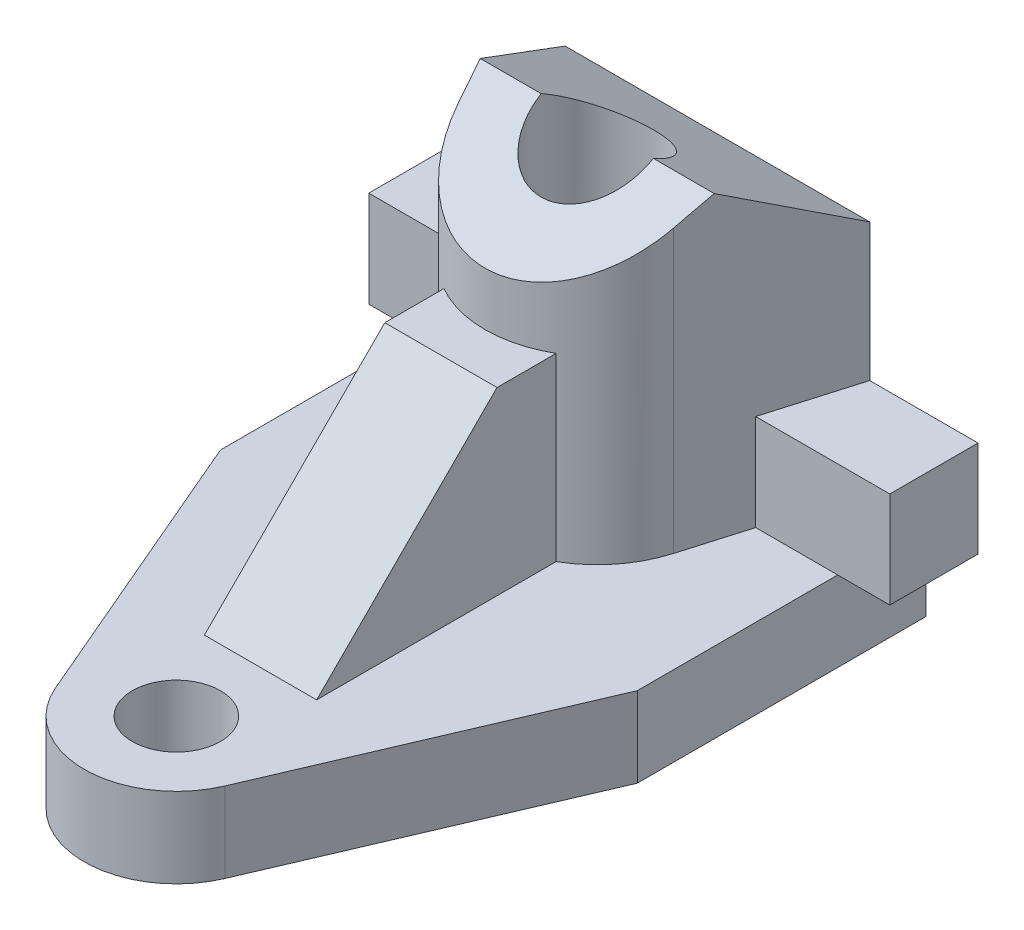
ISO-10303-21;
HEADER;
FILE_DESCRIPTION(('STEP AP214'),'2;1');
FILE_NAME('part.step','',(''),(''),'','','');
FILE_SCHEMA(('AUTOMOTIVE_DESIGN { 1 0 10303 214 1 1 1 1 }'));
ENDSEC;
DATA;
#1=APPLICATION_CONTEXT('core data for automotive mechanical design processes');
#2=APPLICATION_PROTOCOL_DEFINITION('international standard','automotive_design',2000,#1);
#3=PRODUCT_CONTEXT('',#1,'mechanical');
#4=PRODUCT('Part','Part','',(#3));
#5=PRODUCT_RELATED_PRODUCT_CATEGORY('part','',(#4));
#6=PRODUCT_DEFINITION_FORMATION('','',#4);
#7=PRODUCT_DEFINITION_CONTEXT('part definition',#1,'design');
#8=PRODUCT_DEFINITION('design','',#6,#7);
#9=PRODUCT_DEFINITION_SHAPE('','',#8);
#10=(LENGTH_UNIT() NAMED_UNIT(*) SI_UNIT(.MILLI.,.METRE.));
#11=(NAMED_UNIT(*) PLANE_ANGLE_UNIT() SI_UNIT($,.RADIAN.));
#12=(NAMED_UNIT(*) SI_UNIT($,.STERADIAN.) SOLID_ANGLE_UNIT());
#13=UNCERTAINTY_MEASURE_WITH_UNIT(LENGTH_MEASURE(1.E-05),#10,'distance_accuracy_value','');
#14=(GEOMETRIC_REPRESENTATION_CONTEXT(3) GLOBAL_UNCERTAINTY_ASSIGNED_CONTEXT((#13)) GLOBAL_UNIT_ASSIGNED_CONTEXT((#10,
#11,#12)) REPRESENTATION_CONTEXT('',''));
#15=CARTESIAN_POINT('',(0.,0.,0.));
#16=DIRECTION('',(0.,0.,1.));
#17=DIRECTION('',(1.,0.,0.));
#18=AXIS2_PLACEMENT_3D('',#15,#16,#17);
#19=CARTESIAN_POINT('',(0.,47.5,15.));
#20=DIRECTION('',(0.,-1.,0.));
#21=DIRECTION('',(0.,0.,-1.));
#22=AXIS2_PLACEMENT_3D('',#19,#20,#21);
#23=CYLINDRICAL_SURFACE('',#22,14.);
#24=DIRECTION('',(0.,-1.,0.));
#25=VECTOR('',#24,1.);
#26=CARTESIAN_POINT('',(13.432026805815,47.5,18.9472339540324));
#27=LINE('',#26,#25);
#28=CARTESIAN_POINT('',(13.432026805815,45.1417782203444,18.9472339540324));
#29=VERTEX_POINT('',#28);
#30=CARTESIAN_POINT('',(13.432026805815,10.,18.9472339540324));
#31=VERTEX_POINT('',#30);
#32=EDGE_CURVE('E324',#29,#31,#27,.T.);
#33=ORIENTED_EDGE('',*,*,#32,.F.);
#34=CARTESIAN_POINT('',(0.,47.5,15.));
#35=DIRECTION('',(0.,0.858462268371686,0.512876723767164));
#36=DIRECTION('',(0.,-0.512876723767164,0.858462268371686));
#37=AXIS2_PLACEMENT_3D('',#34,#35,#36);
#38=ELLIPSE('',#37,16.3082298614649,14.);
#39=CARTESIAN_POINT('',(-13.432026805815,45.1417782203444,18.9472339540324));
#40=VERTEX_POINT('',#39);
#41=EDGE_CURVE('E286',#40,#29,#38,.T.);
#42=ORIENTED_EDGE('',*,*,#41,.F.);
#43=DIRECTION('',(0.,-1.,0.));
#44=VECTOR('',#43,1.);
#45=CARTESIAN_POINT('',(-13.432026805815,47.5,18.9472339540324));
#46=LINE('',#45,#44);
#47=CARTESIAN_POINT('',(-13.432026805815,10.,18.9472339540324));
#48=VERTEX_POINT('',#47);
#49=EDGE_CURVE('E284',#40,#48,#46,.T.);
#50=ORIENTED_EDGE('',*,*,#49,.T.);
#51=CARTESIAN_POINT('',(0.,10.,15.));
#52=DIRECTION('',(0.,-1.,0.));
#53=DIRECTION('',(0.,0.,-1.));
#54=AXIS2_PLACEMENT_3D('',#51,#52,#53);
#55=CIRCLE('',#54,14.);
#56=CARTESIAN_POINT('',(-7.,10.,27.1243556529821));
#57=VERTEX_POINT('',#56);
#58=EDGE_CURVE('E336',#48,#57,#55,.F.);
#59=ORIENTED_EDGE('',*,*,#58,.T.);
#60=DIRECTION('',(0.,-1.,0.));
#61=VECTOR('',#60,1.);
#62=CARTESIAN_POINT('',(-7.,47.5,27.1243556529821));
#63=LINE('',#62,#61);
#64=CARTESIAN_POINT('',(-7.,32.5,27.1243556529821));
#65=VERTEX_POINT('',#64);
#66=EDGE_CURVE('E438',#57,#65,#63,.F.);
#67=ORIENTED_EDGE('',*,*,#66,.T.);
#68=CARTESIAN_POINT('',(0.,32.5,15.));
#69=DIRECTION('',(0.,-1.,0.));
#70=DIRECTION('',(0.,0.,-1.));
#71=AXIS2_PLACEMENT_3D('',#68,#69,#70);
#72=CIRCLE('',#71,14.);
#73=CARTESIAN_POINT('',(7.,32.5,27.1243556529821));
#74=VERTEX_POINT('',#73);
#75=EDGE_CURVE('E441',#74,#65,#72,.T.);
#76=ORIENTED_EDGE('',*,*,#75,.F.);
#77=DIRECTION('',(0.,-1.,0.));
#78=VECTOR('',#77,1.);
#79=CARTESIAN_POINT('',(7.,47.5,27.1243556529821));
#80=LINE('',#79,#78);
#81=CARTESIAN_POINT('',(7.,10.,27.1243556529821));
#82=VERTEX_POINT('',#81);
#83=EDGE_CURVE('E445',#82,#74,#80,.F.);
#84=ORIENTED_EDGE('',*,*,#83,.F.);
#85=EDGE_CURVE('E340',#82,#31,#55,.F.);
#86=ORIENTED_EDGE('',*,*,#85,.T.);
#87=EDGE_LOOP('',(#33,#42,#50,#59,#67,#76,#84,#86));
#88=FACE_BOUND('',#87,.T.);
#89=ADVANCED_FACE('F111',(#88),#23,.T.);
#90=CARTESIAN_POINT('',(-13.432026805815,47.5,18.9472339540324));
#91=DIRECTION('',(-0.959430486129646,0.,0.281945282430885));
#92=DIRECTION('',(0.281945282430885,0.,0.959430486129646));
#93=AXIS2_PLACEMENT_3D('',#90,#91,#92);
#94=PLANE('',#93);
#95=ORIENTED_EDGE('',*,*,#49,.F.);
#96=DIRECTION('',(-0.244610307501832,0.497296283457055,-0.832383447651177));
#97=VECTOR('',#96,1.);
#98=CARTESIAN_POINT('',(-13.7188898568264,45.724974940818,17.9710688126563));
#99=LINE('',#98,#97);
#100=CARTESIAN_POINT('',(-14.5919899381936,47.5,15.));
#101=VERTEX_POINT('',#100);
#102=EDGE_CURVE('E268',#40,#101,#99,.T.);
#103=ORIENTED_EDGE('',*,*,#102,.T.);
#104=DIRECTION('',(0.248604488500138,0.471722076970145,0.845975230368217));
#105=VECTOR('',#104,1.);
#106=CARTESIAN_POINT('',(-13.6901437947338,49.2112351368513,18.0688886736238));
#107=LINE('',#106,#105);
#108=CARTESIAN_POINT('',(-19.,39.1358884982101,0.));
#109=VERTEX_POINT('',#108);
#110=EDGE_CURVE('E282',#109,#101,#107,.T.);
#111=ORIENTED_EDGE('',*,*,#110,.F.);
#112=DIRECTION('',(0.,-1.,0.));
#113=VECTOR('',#112,1.);
#114=CARTESIAN_POINT('',(-19.,47.5,0.));
#115=LINE('',#114,#113);
#116=CARTESIAN_POINT('',(-19.,22.,0.));
#117=VERTEX_POINT('',#116);
#118=EDGE_CURVE('E322',#109,#117,#115,.T.);
#119=ORIENTED_EDGE('',*,*,#118,.T.);
#120=DIRECTION('',(0.281945282430885,0.,0.959430486129646));
#121=VECTOR('',#120,1.);
#122=CARTESIAN_POINT('',(-17.4896302965844,22.,5.13963108830785));
#123=LINE('',#122,#121);
#124=CARTESIAN_POINT('',(-15.7674592880087,22.,11.));
#125=VERTEX_POINT('',#124);
#126=EDGE_CURVE('E436',#117,#125,#123,.T.);
#127=ORIENTED_EDGE('',*,*,#126,.T.);
#128=DIRECTION('',(0.,1.,0.));
#129=VECTOR('',#128,1.);
#130=CARTESIAN_POINT('',(-15.7674592880087,22.,11.));
#131=LINE('',#130,#129);
#132=CARTESIAN_POINT('',(-15.7674592880087,10.,11.));
#133=VERTEX_POINT('',#132);
#134=EDGE_CURVE('E331',#133,#125,#131,.T.);
#135=ORIENTED_EDGE('',*,*,#134,.F.);
#136=DIRECTION('',(-0.281945282430885,0.,-0.959430486129646));
#137=VECTOR('',#136,1.);
#138=CARTESIAN_POINT('',(0.769585411877711,10.,67.2738439840683));
#139=LINE('',#138,#137);
#140=EDGE_CURVE('E333',#48,#133,#139,.T.);
#141=ORIENTED_EDGE('',*,*,#140,.F.);
#142=EDGE_LOOP('',(#95,#103,#111,#119,#127,#135,#141));
#143=FACE_BOUND('',#142,.T.);
#144=ADVANCED_FACE('F278',(#143),#94,.T.);
#145=CARTESIAN_POINT('',(13.432026805815,47.5,18.9472339540324));
#146=DIRECTION('',(-0.959430486129646,0.,-0.281945282430885));
#147=DIRECTION('',(-0.281945282430885,0.,0.959430486129646));
#148=AXIS2_PLACEMENT_3D('',#145,#146,#147);
#149=PLANE('',#148);
#150=DIRECTION('',(0.244610307501832,0.497296283457055,-0.832383447651177));
#151=VECTOR('',#150,1.);
#152=CARTESIAN_POINT('',(13.7188898568264,45.724974940818,17.9710688126563));
#153=LINE('',#152,#151);
#154=CARTESIAN_POINT('',(14.5919899381936,47.5,15.));
#155=VERTEX_POINT('',#154);
#156=EDGE_CURVE('E452',#29,#155,#153,.T.);
#157=ORIENTED_EDGE('',*,*,#156,.F.);
#158=ORIENTED_EDGE('',*,*,#32,.T.);
#159=DIRECTION('',(0.281945282430885,0.,-0.959430486129646));
#160=VECTOR('',#159,1.);
#161=CARTESIAN_POINT('',(-0.769585411877739,10.,67.2738439840683));
#162=LINE('',#161,#160);
#163=CARTESIAN_POINT('',(15.7674592880086,10.,11.));
#164=VERTEX_POINT('',#163);
#165=EDGE_CURVE('E329',#31,#164,#162,.T.);
#166=ORIENTED_EDGE('',*,*,#165,.T.);
#167=DIRECTION('',(0.,1.,0.));
#168=VECTOR('',#167,1.);
#169=CARTESIAN_POINT('',(15.7674592880086,22.,11.));
#170=LINE('',#169,#168);
#171=CARTESIAN_POINT('',(15.7674592880086,22.,11.));
#172=VERTEX_POINT('',#171);
#173=EDGE_CURVE('E136',#164,#172,#170,.T.);
#174=ORIENTED_EDGE('',*,*,#173,.T.);
#175=DIRECTION('',(-0.281945282430885,0.,0.959430486129646));
#176=VECTOR('',#175,1.);
#177=CARTESIAN_POINT('',(17.4896302965844,22.,5.13963108830785));
#178=LINE('',#177,#176);
#179=CARTESIAN_POINT('',(19.,22.,0.));
#180=VERTEX_POINT('',#179);
#181=EDGE_CURVE('E432',#180,#172,#178,.T.);
#182=ORIENTED_EDGE('',*,*,#181,.F.);
#183=DIRECTION('',(0.,-1.,0.));
#184=VECTOR('',#183,1.);
#185=CARTESIAN_POINT('',(19.,47.5,0.));
#186=LINE('',#185,#184);
#187=CARTESIAN_POINT('',(19.,39.1358884982101,0.));
#188=VERTEX_POINT('',#187);
#189=EDGE_CURVE('E323',#188,#180,#186,.T.);
#190=ORIENTED_EDGE('',*,*,#189,.F.);
#191=DIRECTION('',(-0.248604488500138,0.471722076970145,0.845975230368217));
#192=VECTOR('',#191,1.);
#193=CARTESIAN_POINT('',(13.6901437947338,49.2112351368513,18.0688886736238));
#194=LINE('',#193,#192);
#195=EDGE_CURVE('E293',#188,#155,#194,.T.);
#196=ORIENTED_EDGE('',*,*,#195,.T.);
#197=EDGE_LOOP('',(#157,#158,#166,#174,#182,#190,#196));
#198=FACE_BOUND('',#197,.T.);
#199=ADVANCED_FACE('F460',(#198),#149,.F.);
#200=CARTESIAN_POINT('',(0.,47.5,15.));
#201=DIRECTION('',(0.,-1.,0.));
#202=DIRECTION('',(0.,0.,-1.));
#203=AXIS2_PLACEMENT_3D('',#200,#201,#202);
#204=CYLINDRICAL_SURFACE('',#203,7.);
#205=CARTESIAN_POINT('',(0.,15.,15.));
#206=DIRECTION('',(0.,1.,0.));
#207=DIRECTION('',(0.,0.,1.));
#208=AXIS2_PLACEMENT_3D('',#205,#206,#207);
#209=CIRCLE('',#208,7.);
#210=CARTESIAN_POINT('',(0.,15.,22.));
#211=VERTEX_POINT('',#210);
#212=EDGE_CURVE('E114',#211,#211,#209,.T.);
#213=ORIENTED_EDGE('',*,*,#212,.F.);
#214=EDGE_LOOP('',(#213));
#215=FACE_BOUND('',#214,.T.);
#216=CARTESIAN_POINT('',(0.,47.5,15.));
#217=DIRECTION('',(0.,-0.873395405977944,0.487011770716707));
#218=DIRECTION('',(0.,-0.487011770716707,-0.873395405977944));
#219=AXIS2_PLACEMENT_3D('',#216,#217,#218);
#220=ELLIPSE('',#219,8.01469752655966,7.);
#221=CARTESIAN_POINT('',(-7.,47.5,15.));
#222=VERTEX_POINT('',#221);
#223=CARTESIAN_POINT('',(7.,47.5,15.));
#224=VERTEX_POINT('',#223);
#225=EDGE_CURVE('E300',#222,#224,#220,.T.);
#226=ORIENTED_EDGE('',*,*,#225,.F.);
#227=CARTESIAN_POINT('',(0.,47.5,15.));
#228=DIRECTION('',(0.,0.858462268371686,0.512876723767164));
#229=DIRECTION('',(0.,-0.512876723767164,0.858462268371686));
#230=AXIS2_PLACEMENT_3D('',#227,#228,#229);
#231=ELLIPSE('',#230,8.15411493073244,7.);
#232=EDGE_CURVE('E275',#222,#224,#231,.T.);
#233=ORIENTED_EDGE('',*,*,#232,.T.);
#234=EDGE_LOOP('',(#226,#233));
#235=FACE_BOUND('',#234,.T.);
#236=ADVANCED_FACE('F448',(#215,#235),#204,.F.);
#237=CARTESIAN_POINT('',(-26.,10.,0.));
#238=DIRECTION('',(0.,0.,-1.));
#239=DIRECTION('',(-1.,0.,0.));
#240=AXIS2_PLACEMENT_3D('',#237,#238,#239);
#241=PLANE('',#240);
#242=ORIENTED_EDGE('',*,*,#118,.F.);
#243=DIRECTION('',(1.,0.,0.));
#244=VECTOR('',#243,1.);
#245=CARTESIAN_POINT('',(-32.5,39.1358884982101,0.));
#246=LINE('',#245,#244);
#247=EDGE_CURVE('E281',#109,#188,#246,.T.);
#248=ORIENTED_EDGE('',*,*,#247,.T.);
#249=ORIENTED_EDGE('',*,*,#189,.T.);
#250=DIRECTION('',(-1.,0.,0.));
#251=VECTOR('',#250,1.);
#252=CARTESIAN_POINT('',(-32.5,22.,0.));
#253=LINE('',#252,#251);
#254=CARTESIAN_POINT('',(32.5,22.,0.));
#255=VERTEX_POINT('',#254);
#256=EDGE_CURVE('E352',#255,#180,#253,.T.);
#257=ORIENTED_EDGE('',*,*,#256,.F.);
#258=DIRECTION('',(0.,-1.,0.));
#259=VECTOR('',#258,1.);
#260=CARTESIAN_POINT('',(32.5,22.,0.));
#261=LINE('',#260,#259);
#262=CARTESIAN_POINT('',(32.5,10.,0.));
#263=VERTEX_POINT('',#262);
#264=EDGE_CURVE('E375',#255,#263,#261,.T.);
#265=ORIENTED_EDGE('',*,*,#264,.T.);
#266=DIRECTION('',(-1.,0.,0.));
#267=VECTOR('',#266,1.);
#268=CARTESIAN_POINT('',(-32.5,10.,0.));
#269=LINE('',#268,#267);
#270=CARTESIAN_POINT('',(26.,10.,0.));
#271=VERTEX_POINT('',#270);
#272=EDGE_CURVE('E347',#263,#271,#269,.T.);
#273=ORIENTED_EDGE('',*,*,#272,.T.);
#274=DIRECTION('',(0.,-1.,0.));
#275=VECTOR('',#274,1.);
#276=CARTESIAN_POINT('',(26.,10.,0.));
#277=LINE('',#276,#275);
#278=CARTESIAN_POINT('',(26.,0.,0.));
#279=VERTEX_POINT('',#278);
#280=EDGE_CURVE('E422',#271,#279,#277,.T.);
#281=ORIENTED_EDGE('',*,*,#280,.T.);
#282=DIRECTION('',(1.,0.,0.));
#283=VECTOR('',#282,1.);
#284=CARTESIAN_POINT('',(-26.,0.,0.));
#285=LINE('',#284,#283);
#286=CARTESIAN_POINT('',(-26.,0.,0.));
#287=VERTEX_POINT('',#286);
#288=EDGE_CURVE('E418',#287,#279,#285,.T.);
#289=ORIENTED_EDGE('',*,*,#288,.F.);
#290=DIRECTION('',(0.,-1.,0.));
#291=VECTOR('',#290,1.);
#292=CARTESIAN_POINT('',(-26.,10.,0.));
#293=LINE('',#292,#291);
#294=CARTESIAN_POINT('',(-26.,10.,0.));
#295=VERTEX_POINT('',#294);
#296=EDGE_CURVE('E404',#295,#287,#293,.T.);
#297=ORIENTED_EDGE('',*,*,#296,.F.);
#298=CARTESIAN_POINT('',(-32.5,10.,0.));
#299=VERTEX_POINT('',#298);
#300=EDGE_CURVE('E370',#295,#299,#269,.T.);
#301=ORIENTED_EDGE('',*,*,#300,.T.);
#302=DIRECTION('',(0.,-1.,0.));
#303=VECTOR('',#302,1.);
#304=CARTESIAN_POINT('',(-32.5,22.,0.));
#305=LINE('',#304,#303);
#306=CARTESIAN_POINT('',(-32.5,22.,0.));
#307=VERTEX_POINT('',#306);
#308=EDGE_CURVE('E358',#307,#299,#305,.T.);
#309=ORIENTED_EDGE('',*,*,#308,.F.);
#310=EDGE_CURVE('E355',#117,#307,#253,.T.);
#311=ORIENTED_EDGE('',*,*,#310,.F.);
#312=EDGE_LOOP('',(#242,#248,#249,#257,#265,#273,#281,#289,#297,#301,#309,#311));
#313=FACE_BOUND('',#312,.T.);
#314=ADVANCED_FACE('F479',(#313),#241,.T.);
#315=CARTESIAN_POINT('',(0.,10.,67.5));
#316=DIRECTION('',(0.,-1.,0.));
#317=DIRECTION('',(0.,0.,-1.));
#318=AXIS2_PLACEMENT_3D('',#315,#316,#317);
#319=PLANE('',#318);
#320=DIRECTION('',(-1.,0.,0.));
#321=VECTOR('',#320,1.);
#322=CARTESIAN_POINT('',(7.,10.,57.));
#323=LINE('',#322,#321);
#324=CARTESIAN_POINT('',(7.,10.,57.));
#325=VERTEX_POINT('',#324);
#326=CARTESIAN_POINT('',(-7.,10.,57.));
#327=VERTEX_POINT('',#326);
#328=EDGE_CURVE('E309',#325,#327,#323,.T.);
#329=ORIENTED_EDGE('',*,*,#328,.T.);
#330=DIRECTION('',(0.,0.,-1.));
#331=VECTOR('',#330,1.);
#332=CARTESIAN_POINT('',(-7.,10.,26.5));
#333=LINE('',#332,#331);
#334=EDGE_CURVE('E311',#327,#57,#333,.T.);
#335=ORIENTED_EDGE('',*,*,#334,.T.);
#336=ORIENTED_EDGE('',*,*,#58,.F.);
#337=ORIENTED_EDGE('',*,*,#140,.T.);
#338=DIRECTION('',(1.,0.,0.));
#339=VECTOR('',#338,1.);
#340=CARTESIAN_POINT('',(-32.5,10.,11.));
#341=LINE('',#340,#339);
#342=CARTESIAN_POINT('',(-26.,10.,11.));
#343=VERTEX_POINT('',#342);
#344=EDGE_CURVE('E362',#343,#133,#341,.T.);
#345=ORIENTED_EDGE('',*,*,#344,.F.);
#346=DIRECTION('',(0.,0.,1.));
#347=VECTOR('',#346,1.);
#348=CARTESIAN_POINT('',(-26.,10.,0.));
#349=LINE('',#348,#347);
#350=CARTESIAN_POINT('',(-26.,10.,36.));
#351=VERTEX_POINT('',#350);
#352=EDGE_CURVE('E395',#343,#351,#349,.T.);
#353=ORIENTED_EDGE('',*,*,#352,.T.);
#354=DIRECTION('',(0.393668654576833,0.,0.919252408429625));
#355=VECTOR('',#354,1.);
#356=CARTESIAN_POINT('',(-26.,10.,36.));
#357=LINE('',#356,#355);
#358=CARTESIAN_POINT('',(-10.5714026969407,10.,72.0271895276336));
#359=VERTEX_POINT('',#358);
#360=EDGE_CURVE('E392',#351,#359,#357,.T.);
#361=ORIENTED_EDGE('',*,*,#360,.T.);
#362=CARTESIAN_POINT('',(0.,10.,67.5));
#363=DIRECTION('',(0.,-1.,0.));
#364=DIRECTION('',(0.,0.,-1.));
#365=AXIS2_PLACEMENT_3D('',#362,#363,#364);
#366=CIRCLE('',#365,11.5);
#367=CARTESIAN_POINT('',(10.5714026969407,10.,72.0271895276336));
#368=VERTEX_POINT('',#367);
#369=EDGE_CURVE('E394',#368,#359,#366,.T.);
#370=ORIENTED_EDGE('',*,*,#369,.F.);
#371=DIRECTION('',(-0.393668654576833,0.,0.919252408429625));
#372=VECTOR('',#371,1.);
#373=CARTESIAN_POINT('',(26.,10.,36.));
#374=LINE('',#373,#372);
#375=CARTESIAN_POINT('',(26.,10.,36.));
#376=VERTEX_POINT('',#375);
#377=EDGE_CURVE('E400',#376,#368,#374,.T.);
#378=ORIENTED_EDGE('',*,*,#377,.F.);
#379=DIRECTION('',(0.,0.,1.));
#380=VECTOR('',#379,1.);
#381=CARTESIAN_POINT('',(26.,10.,0.));
#382=LINE('',#381,#380);
#383=CARTESIAN_POINT('',(26.,10.,11.));
#384=VERTEX_POINT('',#383);
#385=EDGE_CURVE('E399',#384,#376,#382,.T.);
#386=ORIENTED_EDGE('',*,*,#385,.F.);
#387=EDGE_CURVE('E364',#164,#384,#341,.T.);
#388=ORIENTED_EDGE('',*,*,#387,.F.);
#389=ORIENTED_EDGE('',*,*,#165,.F.);
#390=ORIENTED_EDGE('',*,*,#85,.F.);
#391=DIRECTION('',(0.,0.,-1.));
#392=VECTOR('',#391,1.);
#393=CARTESIAN_POINT('',(7.,10.,26.5));
#394=LINE('',#393,#392);
#395=EDGE_CURVE('E303',#325,#82,#394,.T.);
#396=ORIENTED_EDGE('',*,*,#395,.F.);
#397=EDGE_LOOP('',(#329,#335,#336,#337,#345,#353,#361,#370,#378,#386,#388,#389,#390,#396));
#398=FACE_BOUND('',#397,.T.);
#399=CARTESIAN_POINT('',(0.,10.,67.5));
#400=DIRECTION('',(0.,-1.,0.));
#401=DIRECTION('',(0.,0.,-1.));
#402=AXIS2_PLACEMENT_3D('',#399,#400,#401);
#403=CIRCLE('',#402,5.5);
#404=CARTESIAN_POINT('',(0.,10.,62.));
#405=VERTEX_POINT('',#404);
#406=EDGE_CURVE('E385',#405,#405,#403,.T.);
#407=ORIENTED_EDGE('',*,*,#406,.T.);
#408=EDGE_LOOP('',(#407));
#409=FACE_BOUND('',#408,.T.);
#410=ADVANCED_FACE('F467',(#398,#409),#319,.F.);
#411=CARTESIAN_POINT('',(-32.5,22.,11.));
#412=DIRECTION('',(0.,0.,-1.));
#413=DIRECTION('',(-1.,0.,0.));
#414=AXIS2_PLACEMENT_3D('',#411,#412,#413);
#415=PLANE('',#414);
#416=ORIENTED_EDGE('',*,*,#173,.F.);
#417=ORIENTED_EDGE('',*,*,#387,.T.);
#418=CARTESIAN_POINT('',(32.5,10.,11.));
#419=VERTEX_POINT('',#418);
#420=EDGE_CURVE('E360',#384,#419,#341,.T.);
#421=ORIENTED_EDGE('',*,*,#420,.T.);
#422=DIRECTION('',(0.,-1.,0.));
#423=VECTOR('',#422,1.);
#424=CARTESIAN_POINT('',(32.5,22.,11.));
#425=LINE('',#424,#423);
#426=CARTESIAN_POINT('',(32.5,22.,11.));
#427=VERTEX_POINT('',#426);
#428=EDGE_CURVE('E374',#427,#419,#425,.T.);
#429=ORIENTED_EDGE('',*,*,#428,.F.);
#430=DIRECTION('',(1.,0.,0.));
#431=VECTOR('',#430,1.);
#432=CARTESIAN_POINT('',(-32.5,22.,11.));
#433=LINE('',#432,#431);
#434=EDGE_CURVE('E343',#172,#427,#433,.T.);
#435=ORIENTED_EDGE('',*,*,#434,.F.);
#436=EDGE_LOOP('',(#416,#417,#421,#429,#435));
#437=FACE_BOUND('',#436,.T.);
#438=ADVANCED_FACE('F472',(#437),#415,.F.);
#439=ORIENTED_EDGE('',*,*,#344,.T.);
#440=ORIENTED_EDGE('',*,*,#134,.T.);
#441=CARTESIAN_POINT('',(-32.5,22.,11.));
#442=VERTEX_POINT('',#441);
#443=EDGE_CURVE('E350',#442,#125,#433,.T.);
#444=ORIENTED_EDGE('',*,*,#443,.F.);
#445=DIRECTION('',(0.,-1.,0.));
#446=VECTOR('',#445,1.);
#447=CARTESIAN_POINT('',(-32.5,22.,11.));
#448=LINE('',#447,#446);
#449=CARTESIAN_POINT('',(-32.5,10.,11.));
#450=VERTEX_POINT('',#449);
#451=EDGE_CURVE('E377',#442,#450,#448,.T.);
#452=ORIENTED_EDGE('',*,*,#451,.T.);
#453=EDGE_CURVE('E359',#450,#343,#341,.T.);
#454=ORIENTED_EDGE('',*,*,#453,.T.);
#455=EDGE_LOOP('',(#439,#440,#444,#452,#454));
#456=FACE_BOUND('',#455,.T.);
#457=ADVANCED_FACE('F490',(#456),#415,.F.);
#458=CARTESIAN_POINT('',(0.,22.,0.));
#459=DIRECTION('',(0.,1.,0.));
#460=DIRECTION('',(0.,0.,1.));
#461=AXIS2_PLACEMENT_3D('',#458,#459,#460);
#462=PLANE('',#461);
#463=ORIENTED_EDGE('',*,*,#126,.F.);
#464=ORIENTED_EDGE('',*,*,#310,.T.);
#465=DIRECTION('',(0.,0.,1.));
#466=VECTOR('',#465,1.);
#467=CARTESIAN_POINT('',(-32.5,22.,0.));
#468=LINE('',#467,#466);
#469=EDGE_CURVE('E345',#307,#442,#468,.T.);
#470=ORIENTED_EDGE('',*,*,#469,.T.);
#471=ORIENTED_EDGE('',*,*,#443,.T.);
#472=EDGE_LOOP('',(#463,#464,#470,#471));
#473=FACE_BOUND('',#472,.T.);
#474=ADVANCED_FACE('F483',(#473),#462,.T.);
#475=CARTESIAN_POINT('',(-26.,10.,0.));
#476=DIRECTION('',(1.,0.,0.));
#477=DIRECTION('',(0.,0.,-1.));
#478=AXIS2_PLACEMENT_3D('',#475,#476,#477);
#479=PLANE('',#478);
#480=DIRECTION('',(0.,0.,1.));
#481=VECTOR('',#480,1.);
#482=CARTESIAN_POINT('',(-26.,0.,0.));
#483=LINE('',#482,#481);
#484=CARTESIAN_POINT('',(-26.,0.,36.));
#485=VERTEX_POINT('',#484);
#486=EDGE_CURVE('E383',#287,#485,#483,.T.);
#487=ORIENTED_EDGE('',*,*,#486,.T.);
#488=DIRECTION('',(0.,-1.,0.));
#489=VECTOR('',#488,1.);
#490=CARTESIAN_POINT('',(-26.,10.,36.));
#491=LINE('',#490,#489);
#492=EDGE_CURVE('E431',#351,#485,#491,.T.);
#493=ORIENTED_EDGE('',*,*,#492,.F.);
#494=ORIENTED_EDGE('',*,*,#352,.F.);
#495=EDGE_CURVE('E389',#295,#343,#349,.T.);
#496=ORIENTED_EDGE('',*,*,#495,.F.);
#497=ORIENTED_EDGE('',*,*,#296,.T.);
#498=EDGE_LOOP('',(#487,#493,#494,#496,#497));
#499=FACE_BOUND('',#498,.T.);
#500=ADVANCED_FACE('F113',(#499),#479,.F.);
#501=CARTESIAN_POINT('',(-26.,10.,36.));
#502=DIRECTION('',(0.919252408429625,0.,-0.393668654576833));
#503=DIRECTION('',(-0.393668654576833,0.,-0.919252408429625));
#504=AXIS2_PLACEMENT_3D('',#501,#502,#503);
#505=PLANE('',#504);
#506=DIRECTION('',(0.393668654576833,0.,0.919252408429625));
#507=VECTOR('',#506,1.);
#508=CARTESIAN_POINT('',(-26.,0.,36.));
#509=LINE('',#508,#507);
#510=CARTESIAN_POINT('',(-10.5714026969407,0.,72.0271895276336));
#511=VERTEX_POINT('',#510);
#512=EDGE_CURVE('E410',#485,#511,#509,.T.);
#513=ORIENTED_EDGE('',*,*,#512,.T.);
#514=DIRECTION('',(0.,-1.,0.));
#515=VECTOR('',#514,1.);
#516=CARTESIAN_POINT('',(-10.5714026969407,10.,72.0271895276336));
#517=LINE('',#516,#515);
#518=EDGE_CURVE('E429',#359,#511,#517,.T.);
#519=ORIENTED_EDGE('',*,*,#518,.F.);
#520=ORIENTED_EDGE('',*,*,#360,.F.);
#521=ORIENTED_EDGE('',*,*,#492,.T.);
#522=EDGE_LOOP('',(#513,#519,#520,#521));
#523=FACE_BOUND('',#522,.T.);
#524=ADVANCED_FACE('F557',(#523),#505,.F.);
#525=CARTESIAN_POINT('',(0.,10.,67.5));
#526=DIRECTION('',(0.,-1.,0.));
#527=DIRECTION('',(0.,0.,-1.));
#528=AXIS2_PLACEMENT_3D('',#525,#526,#527);
#529=CYLINDRICAL_SURFACE('',#528,11.5);
#530=CARTESIAN_POINT('',(0.,0.,67.5));
#531=DIRECTION('',(0.,-1.,0.));
#532=DIRECTION('',(0.,0.,-1.));
#533=AXIS2_PLACEMENT_3D('',#530,#531,#532);
#534=CIRCLE('',#533,11.5);
#535=CARTESIAN_POINT('',(10.5714026969407,0.,72.0271895276336));
#536=VERTEX_POINT('',#535);
#537=EDGE_CURVE('E408',#536,#511,#534,.T.);
#538=ORIENTED_EDGE('',*,*,#537,.F.);
#539=DIRECTION('',(0.,-1.,0.));
#540=VECTOR('',#539,1.);
#541=CARTESIAN_POINT('',(10.5714026969407,10.,72.0271895276336));
#542=LINE('',#541,#540);
#543=EDGE_CURVE('E430',#368,#536,#542,.T.);
#544=ORIENTED_EDGE('',*,*,#543,.F.);
#545=ORIENTED_EDGE('',*,*,#369,.T.);
#546=ORIENTED_EDGE('',*,*,#518,.T.);
#547=EDGE_LOOP('',(#538,#544,#545,#546));
#548=FACE_BOUND('',#547,.T.);
#549=ADVANCED_FACE('F560',(#548),#529,.T.);
#550=CARTESIAN_POINT('',(26.,10.,36.));
#551=DIRECTION('',(0.919252408429625,0.,0.393668654576833));
#552=DIRECTION('',(0.393668654576833,0.,-0.919252408429625));
#553=AXIS2_PLACEMENT_3D('',#550,#551,#552);
#554=PLANE('',#553);
#555=DIRECTION('',(-0.393668654576833,0.,0.919252408429625));
#556=VECTOR('',#555,1.);
#557=CARTESIAN_POINT('',(26.,0.,36.));
#558=LINE('',#557,#556);
#559=CARTESIAN_POINT('',(26.,0.,36.));
#560=VERTEX_POINT('',#559);
#561=EDGE_CURVE('E413',#560,#536,#558,.T.);
#562=ORIENTED_EDGE('',*,*,#561,.F.);
#563=DIRECTION('',(0.,-1.,0.));
#564=VECTOR('',#563,1.);
#565=CARTESIAN_POINT('',(26.,10.,36.));
#566=LINE('',#565,#564);
#567=EDGE_CURVE('E424',#376,#560,#566,.T.);
#568=ORIENTED_EDGE('',*,*,#567,.F.);
#569=ORIENTED_EDGE('',*,*,#377,.T.);
#570=ORIENTED_EDGE('',*,*,#543,.T.);
#571=EDGE_LOOP('',(#562,#568,#569,#570));
#572=FACE_BOUND('',#571,.T.);
#573=ADVANCED_FACE('F551',(#572),#554,.T.);
#574=CARTESIAN_POINT('',(26.,10.,0.));
#575=DIRECTION('',(1.,0.,0.));
#576=DIRECTION('',(0.,0.,-1.));
#577=AXIS2_PLACEMENT_3D('',#574,#575,#576);
#578=PLANE('',#577);
#579=DIRECTION('',(0.,0.,1.));
#580=VECTOR('',#579,1.);
#581=CARTESIAN_POINT('',(26.,0.,0.));
#582=LINE('',#581,#580);
#583=EDGE_CURVE('E416',#279,#560,#582,.T.);
#584=ORIENTED_EDGE('',*,*,#583,.F.);
#585=ORIENTED_EDGE('',*,*,#280,.F.);
#586=EDGE_CURVE('E402',#271,#384,#382,.T.);
#587=ORIENTED_EDGE('',*,*,#586,.T.);
#588=ORIENTED_EDGE('',*,*,#385,.T.);
#589=ORIENTED_EDGE('',*,*,#567,.T.);
#590=EDGE_LOOP('',(#584,#585,#587,#588,#589));
#591=FACE_BOUND('',#590,.T.);
#592=ADVANCED_FACE('F550',(#591),#578,.T.);
#593=CARTESIAN_POINT('',(0.,0.,67.5));
#594=DIRECTION('',(0.,-1.,0.));
#595=DIRECTION('',(0.,0.,-1.));
#596=AXIS2_PLACEMENT_3D('',#593,#594,#595);
#597=PLANE('',#596);
#598=CARTESIAN_POINT('',(0.,0.,15.));
#599=DIRECTION('',(0.,1.,0.));
#600=DIRECTION('',(0.,0.,1.));
#601=AXIS2_PLACEMENT_3D('',#598,#599,#600);
#602=CIRCLE('',#601,10.);
#603=CARTESIAN_POINT('',(0.,0.,25.));
#604=VERTEX_POINT('',#603);
#605=EDGE_CURVE('E289',#604,#604,#602,.T.);
#606=ORIENTED_EDGE('',*,*,#605,.T.);
#607=EDGE_LOOP('',(#606));
#608=FACE_BOUND('',#607,.T.);
#609=ORIENTED_EDGE('',*,*,#288,.T.);
#610=ORIENTED_EDGE('',*,*,#583,.T.);
#611=ORIENTED_EDGE('',*,*,#561,.T.);
#612=ORIENTED_EDGE('',*,*,#537,.T.);
#613=ORIENTED_EDGE('',*,*,#512,.F.);
#614=ORIENTED_EDGE('',*,*,#486,.F.);
#615=EDGE_LOOP('',(#609,#610,#611,#612,#613,#614));
#616=FACE_BOUND('',#615,.T.);
#617=CARTESIAN_POINT('',(0.,0.,67.5));
#618=DIRECTION('',(0.,-1.,0.));
#619=DIRECTION('',(0.,0.,-1.));
#620=AXIS2_PLACEMENT_3D('',#617,#618,#619);
#621=CIRCLE('',#620,5.5);
#622=CARTESIAN_POINT('',(0.,0.,62.));
#623=VERTEX_POINT('',#622);
#624=EDGE_CURVE('E382',#623,#623,#621,.T.);
#625=ORIENTED_EDGE('',*,*,#624,.F.);
#626=EDGE_LOOP('',(#625));
#627=FACE_BOUND('',#626,.T.);
#628=ADVANCED_FACE('F545',(#608,#616,#627),#597,.T.);
#629=CARTESIAN_POINT('',(0.,10.,67.5));
#630=DIRECTION('',(0.,-1.,0.));
#631=DIRECTION('',(0.,0.,-1.));
#632=AXIS2_PLACEMENT_3D('',#629,#630,#631);
#633=CYLINDRICAL_SURFACE('',#632,5.5);
#634=ORIENTED_EDGE('',*,*,#406,.F.);
#635=EDGE_LOOP('',(#634));
#636=FACE_BOUND('',#635,.T.);
#637=ORIENTED_EDGE('',*,*,#624,.T.);
#638=EDGE_LOOP('',(#637));
#639=FACE_BOUND('',#638,.T.);
#640=ADVANCED_FACE('F536',(#636,#639),#633,.F.);
#641=CARTESIAN_POINT('',(0.,10.,0.));
#642=DIRECTION('',(0.,1.,0.));
#643=DIRECTION('',(0.,0.,1.));
#644=AXIS2_PLACEMENT_3D('',#641,#642,#643);
#645=PLANE('',#644);
#646=ORIENTED_EDGE('',*,*,#300,.F.);
#647=ORIENTED_EDGE('',*,*,#495,.T.);
#648=ORIENTED_EDGE('',*,*,#453,.F.);
#649=DIRECTION('',(0.,0.,1.));
#650=VECTOR('',#649,1.);
#651=CARTESIAN_POINT('',(-32.5,10.,0.));
#652=LINE('',#651,#650);
#653=EDGE_CURVE('E342',#299,#450,#652,.T.);
#654=ORIENTED_EDGE('',*,*,#653,.F.);
#655=EDGE_LOOP('',(#646,#647,#648,#654));
#656=FACE_BOUND('',#655,.T.);
#657=ADVANCED_FACE('F514',(#656),#645,.F.);
#658=CARTESIAN_POINT('',(-32.5,22.,0.));
#659=DIRECTION('',(1.,0.,0.));
#660=DIRECTION('',(0.,0.,-1.));
#661=AXIS2_PLACEMENT_3D('',#658,#659,#660);
#662=PLANE('',#661);
#663=ORIENTED_EDGE('',*,*,#653,.T.);
#664=ORIENTED_EDGE('',*,*,#451,.F.);
#665=ORIENTED_EDGE('',*,*,#469,.F.);
#666=ORIENTED_EDGE('',*,*,#308,.T.);
#667=EDGE_LOOP('',(#663,#664,#665,#666));
#668=FACE_BOUND('',#667,.T.);
#669=ADVANCED_FACE('F535',(#668),#662,.F.);
#670=CARTESIAN_POINT('',(32.5,22.,0.));
#671=DIRECTION('',(-1.,0.,0.));
#672=DIRECTION('',(0.,0.,1.));
#673=AXIS2_PLACEMENT_3D('',#670,#671,#672);
#674=PLANE('',#673);
#675=DIRECTION('',(0.,0.,-1.));
#676=VECTOR('',#675,1.);
#677=CARTESIAN_POINT('',(32.5,10.,0.));
#678=LINE('',#677,#676);
#679=EDGE_CURVE('E361',#419,#263,#678,.T.);
#680=ORIENTED_EDGE('',*,*,#679,.T.);
#681=ORIENTED_EDGE('',*,*,#264,.F.);
#682=DIRECTION('',(0.,0.,-1.));
#683=VECTOR('',#682,1.);
#684=CARTESIAN_POINT('',(32.5,22.,0.));
#685=LINE('',#684,#683);
#686=EDGE_CURVE('E346',#427,#255,#685,.T.);
#687=ORIENTED_EDGE('',*,*,#686,.F.);
#688=ORIENTED_EDGE('',*,*,#428,.T.);
#689=EDGE_LOOP('',(#680,#681,#687,#688));
#690=FACE_BOUND('',#689,.T.);
#691=ADVANCED_FACE('F527',(#690),#674,.F.);
#692=ORIENTED_EDGE('',*,*,#256,.T.);
#693=ORIENTED_EDGE('',*,*,#181,.T.);
#694=ORIENTED_EDGE('',*,*,#434,.T.);
#695=ORIENTED_EDGE('',*,*,#686,.T.);
#696=EDGE_LOOP('',(#692,#693,#694,#695));
#697=FACE_BOUND('',#696,.T.);
#698=ADVANCED_FACE('F473',(#697),#462,.T.);
#699=ORIENTED_EDGE('',*,*,#586,.F.);
#700=ORIENTED_EDGE('',*,*,#272,.F.);
#701=ORIENTED_EDGE('',*,*,#679,.F.);
#702=ORIENTED_EDGE('',*,*,#420,.F.);
#703=EDGE_LOOP('',(#699,#700,#701,#702));
#704=FACE_BOUND('',#703,.T.);
#705=ADVANCED_FACE('F503',(#704),#645,.F.);
#706=CARTESIAN_POINT('',(7.,0.,0.));
#707=DIRECTION('',(-1.,0.,0.));
#708=DIRECTION('',(0.,0.,1.));
#709=AXIS2_PLACEMENT_3D('',#706,#707,#708);
#710=PLANE('',#709);
#711=ORIENTED_EDGE('',*,*,#395,.T.);
#712=ORIENTED_EDGE('',*,*,#83,.T.);
#713=DIRECTION('',(0.,0.,1.));
#714=VECTOR('',#713,1.);
#715=CARTESIAN_POINT('',(7.,32.5,26.5));
#716=LINE('',#715,#714);
#717=CARTESIAN_POINT('',(7.,32.5,34.5000000000001));
#718=VERTEX_POINT('',#717);
#719=EDGE_CURVE('E304',#74,#718,#716,.T.);
#720=ORIENTED_EDGE('',*,*,#719,.T.);
#721=DIRECTION('',(0.,-0.707106781186549,0.707106781186546));
#722=VECTOR('',#721,1.);
#723=CARTESIAN_POINT('',(7.,32.5,34.5000000000001));
#724=LINE('',#723,#722);
#725=EDGE_CURVE('E308',#718,#325,#724,.T.);
#726=ORIENTED_EDGE('',*,*,#725,.T.);
#727=EDGE_LOOP('',(#711,#712,#720,#726));
#728=FACE_BOUND('',#727,.T.);
#729=ADVANCED_FACE('F501',(#728),#710,.F.);
#730=CARTESIAN_POINT('',(-7.,0.,0.));
#731=DIRECTION('',(-1.,0.,0.));
#732=DIRECTION('',(0.,0.,1.));
#733=AXIS2_PLACEMENT_3D('',#730,#731,#732);
#734=PLANE('',#733);
#735=ORIENTED_EDGE('',*,*,#66,.F.);
#736=ORIENTED_EDGE('',*,*,#334,.F.);
#737=DIRECTION('',(0.,-0.707106781186549,0.707106781186546));
#738=VECTOR('',#737,1.);
#739=CARTESIAN_POINT('',(-7.,32.5,34.5000000000001));
#740=LINE('',#739,#738);
#741=CARTESIAN_POINT('',(-7.,32.5,34.5000000000001));
#742=VERTEX_POINT('',#741);
#743=EDGE_CURVE('E306',#742,#327,#740,.T.);
#744=ORIENTED_EDGE('',*,*,#743,.F.);
#745=DIRECTION('',(0.,0.,1.));
#746=VECTOR('',#745,1.);
#747=CARTESIAN_POINT('',(-7.,32.5,26.5));
#748=LINE('',#747,#746);
#749=EDGE_CURVE('E129',#65,#742,#748,.T.);
#750=ORIENTED_EDGE('',*,*,#749,.F.);
#751=EDGE_LOOP('',(#735,#736,#744,#750));
#752=FACE_BOUND('',#751,.T.);
#753=ADVANCED_FACE('F491',(#752),#734,.T.);
#754=CARTESIAN_POINT('',(7.,32.5,26.5));
#755=DIRECTION('',(0.,-1.,0.));
#756=DIRECTION('',(0.,0.,-1.));
#757=AXIS2_PLACEMENT_3D('',#754,#755,#756);
#758=PLANE('',#757);
#759=ORIENTED_EDGE('',*,*,#719,.F.);
#760=ORIENTED_EDGE('',*,*,#75,.T.);
#761=ORIENTED_EDGE('',*,*,#749,.T.);
#762=DIRECTION('',(-1.,0.,0.));
#763=VECTOR('',#762,1.);
#764=CARTESIAN_POINT('',(7.,32.5,34.5000000000001));
#765=LINE('',#764,#763);
#766=EDGE_CURVE('E319',#718,#742,#765,.T.);
#767=ORIENTED_EDGE('',*,*,#766,.F.);
#768=EDGE_LOOP('',(#759,#760,#761,#767));
#769=FACE_BOUND('',#768,.T.);
#770=ADVANCED_FACE('F499',(#769),#758,.F.);
#771=CARTESIAN_POINT('',(7.,32.5,34.5000000000001));
#772=DIRECTION('',(0.,-0.707106781186546,-0.707106781186549));
#773=DIRECTION('',(0.,0.707106781186549,-0.707106781186546));
#774=AXIS2_PLACEMENT_3D('',#771,#772,#773);
#775=PLANE('',#774);
#776=ORIENTED_EDGE('',*,*,#743,.T.);
#777=ORIENTED_EDGE('',*,*,#328,.F.);
#778=ORIENTED_EDGE('',*,*,#725,.F.);
#779=ORIENTED_EDGE('',*,*,#766,.T.);
#780=EDGE_LOOP('',(#776,#777,#778,#779));
#781=FACE_BOUND('',#780,.T.);
#782=ADVANCED_FACE('F500',(#781),#775,.F.);
#783=CARTESIAN_POINT('',(0.,15.,15.));
#784=DIRECTION('',(0.,-1.,0.));
#785=DIRECTION('',(0.,0.,-1.));
#786=AXIS2_PLACEMENT_3D('',#783,#784,#785);
#787=CYLINDRICAL_SURFACE('',#786,10.);
#788=CARTESIAN_POINT('',(0.,15.,15.));
#789=DIRECTION('',(0.,1.,0.));
#790=DIRECTION('',(0.,0.,1.));
#791=AXIS2_PLACEMENT_3D('',#788,#789,#790);
#792=CIRCLE('',#791,10.);
#793=CARTESIAN_POINT('',(0.,15.,25.));
#794=VERTEX_POINT('',#793);
#795=EDGE_CURVE('E295',#794,#794,#792,.T.);
#796=ORIENTED_EDGE('',*,*,#795,.T.);
#797=EDGE_LOOP('',(#796));
#798=FACE_BOUND('',#797,.T.);
#799=ORIENTED_EDGE('',*,*,#605,.F.);
#800=EDGE_LOOP('',(#799));
#801=FACE_BOUND('',#800,.T.);
#802=ADVANCED_FACE('F661',(#798,#801),#787,.F.);
#803=CARTESIAN_POINT('',(0.,15.,15.));
#804=DIRECTION('',(0.,1.,0.));
#805=DIRECTION('',(0.,0.,1.));
#806=AXIS2_PLACEMENT_3D('',#803,#804,#805);
#807=PLANE('',#806);
#808=ORIENTED_EDGE('',*,*,#212,.T.);
#809=EDGE_LOOP('',(#808));
#810=FACE_BOUND('',#809,.T.);
#811=ORIENTED_EDGE('',*,*,#795,.F.);
#812=EDGE_LOOP('',(#811));
#813=FACE_BOUND('',#812,.T.);
#814=ADVANCED_FACE('F675',(#810,#813),#807,.F.);
#815=CARTESIAN_POINT('',(-32.5,47.5,15.));
#816=DIRECTION('',(0.,-0.873395405977944,0.487011770716707));
#817=DIRECTION('',(0.,-0.487011770716707,-0.873395405977944));
#818=AXIS2_PLACEMENT_3D('',#815,#816,#817);
#819=PLANE('',#818);
#820=ORIENTED_EDGE('',*,*,#110,.T.);
#821=DIRECTION('',(1.,0.,0.));
#822=VECTOR('',#821,1.);
#823=CARTESIAN_POINT('',(-32.5,47.5,15.));
#824=LINE('',#823,#822);
#825=EDGE_CURVE('E12',#101,#222,#824,.T.);
#826=ORIENTED_EDGE('',*,*,#825,.T.);
#827=ORIENTED_EDGE('',*,*,#225,.T.);
#828=EDGE_CURVE('E119',#224,#155,#824,.T.);
#829=ORIENTED_EDGE('',*,*,#828,.T.);
#830=ORIENTED_EDGE('',*,*,#195,.F.);
#831=ORIENTED_EDGE('',*,*,#247,.F.);
#832=EDGE_LOOP('',(#820,#826,#827,#829,#830,#831));
#833=FACE_BOUND('',#832,.T.);
#834=ADVANCED_FACE('F287',(#833),#819,.F.);
#835=CARTESIAN_POINT('',(-32.5,41.6097593805513,24.8591905015415));
#836=DIRECTION('',(0.,0.858462268371686,0.512876723767164));
#837=DIRECTION('',(0.,-0.512876723767164,0.858462268371686));
#838=AXIS2_PLACEMENT_3D('',#835,#836,#837);
#839=PLANE('',#838);
#840=ORIENTED_EDGE('',*,*,#41,.T.);
#841=ORIENTED_EDGE('',*,*,#156,.T.);
#842=ORIENTED_EDGE('',*,*,#828,.F.);
#843=ORIENTED_EDGE('',*,*,#232,.F.);
#844=ORIENTED_EDGE('',*,*,#825,.F.);
#845=ORIENTED_EDGE('',*,*,#102,.F.);
#846=EDGE_LOOP('',(#840,#841,#842,#843,#844,#845));
#847=FACE_BOUND('',#846,.T.);
#848=ADVANCED_FACE('F267',(#847),#839,.T.);
#849=CLOSED_SHELL('',(#89,#144,#199,#236,#314,#410,#438,#457,#474,#500,#524,#549,#573,#592,#628,
#640,#657,#669,#691,#698,#705,#729,#753,#770,#782,#802,#814,#834,#848));
#850=MANIFOLD_SOLID_BREP('B2',#849);
#851=ADVANCED_BREP_SHAPE_REPRESENTATION('',(#18,#850),#14);
#852=SHAPE_DEFINITION_REPRESENTATION(#9,#851);
ENDSEC;
END-ISO-10303-21;
